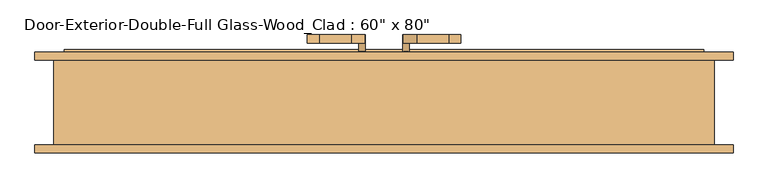
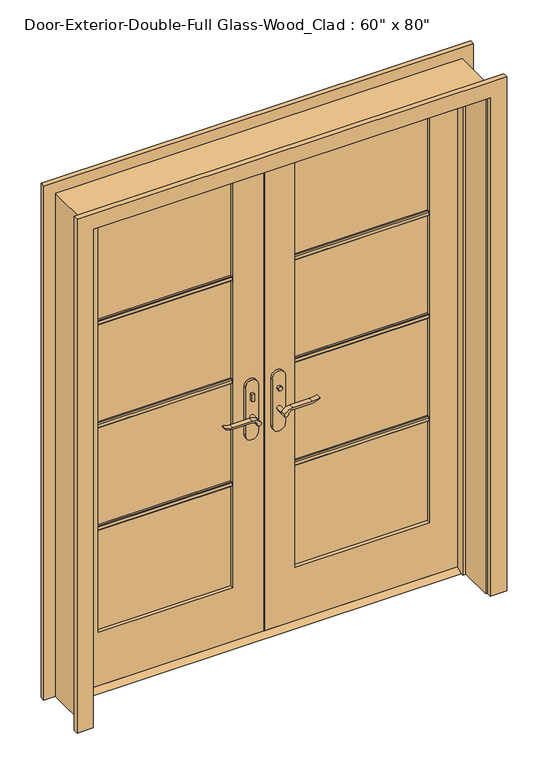
"""IFC4 building model written with IfcOpenShell, lengths in millimetres: door geometry."""

from ifc_helpers import new_model, si_unit, point, frame, frame_2d, origin, place, context, project, spatial, polyline, circle_curve, trimmed, segment, composite_curve, outline, extrude, faceted_brep, source, transform, mapped, element, save


def door_b03bd389(model_context):
    return source(origin(), model_context, "Body", "SolidModel", [
        extrude(outline(polyline([(63.5, 12.7), (98.425, 12.7), (123.825, 0.0), (38.1, 0.0), (63.5, 12.7)])), frame((-762.0, 0.0, 0.0), z_axis=(1.0, 0.0, 0.0), x_axis=(0.0, 1.0, 0.0)), (0.0, 0.0, 1.0), 1524.0),
        extrude(outline(polyline([(-47.4019111, 43.5), (-57.4019111, 43.5), (-57.4019111, 53.5), (-47.4019111, 53.5), (-47.4019111, 43.5)])), frame((0.0, 0.0, 981.9), z_axis=(0.0, 0.0, 1.0), x_axis=(1.0, 0.0, 0.0)), (0.0, 0.0, 1.0), 30.0),
        extrude(outline(composite_curve([segment(trimmed(circle_curve(frame_2d((996.9, -52.4019111)), 8.0), [point((996.9, -60.4019111))], [point((996.9, -44.4019111))], False, "CARTESIAN"), True, "CONTINUOUS"), segment(trimmed(circle_curve(frame_2d((996.9, -52.4019111)), 8.0), [point((996.9, -44.4019111))], [point((996.9, -60.4019111))], False, "CARTESIAN"), True, "CONTINUOUS")], self_intersect=False)), frame((0.0, 108.425, 0.0), z_axis=(0.0, 1.0, 0.0), x_axis=(0.0, 0.0, 1.0)), (0.0, 0.0, 1.0), 10.0),
        extrude(outline(composite_curve([segment(trimmed(circle_curve(frame_2d((897.1555521, -76.0694241)), 37.2832219), [point((919.0523287, -45.8937749))], [point((934.4, -77.7693445))], False, "CARTESIAN"), True, "CONTINUOUS"), segment(polyline([(934.4, -77.7693445), (934.4, -154.045502)]), True, "CONTINUOUS"), segment(trimmed(circle_curve(frame_2d((1017.6850638, -153.9791202)), 83.2850902), [point((934.4, -154.045502))], [point((939.4, -182.4019111))], True, "CARTESIAN"), True, "CONTINUOUS"), segment(polyline([(939.4, -182.4019111), (936.6135558, -182.4019111)]), True, "CONTINUOUS"), segment(trimmed(circle_curve(frame_2d((986.6709207, -150.4622499)), 59.3791355), [point((936.6135558, -182.4019111))], [point((927.4, -154.045502))], False, "CARTESIAN"), True, "CONTINUOUS"), segment(polyline([(927.4, -154.045502), (927.4, -77.7881013)]), True, "CONTINUOUS"), segment(trimmed(circle_curve(frame_2d((909.2738613, -77.7881013)), 18.1261387), [point((927.4, -77.7881013))], [point((914.4, -60.4019111))], True, "CARTESIAN"), True, "CONTINUOUS"), segment(trimmed(circle_curve(frame_2d((914.4, -52.4019111)), 8.0), [point((914.4, -60.4019111))], [point((919.0523287, -45.8937749))], False, "CARTESIAN"), True, "CONTINUOUS")], self_intersect=False)), frame((0.0, 3.5, 0.0), z_axis=(0.0, 1.0, 0.0), x_axis=(0.0, 0.0, 1.0)), (0.0, 0.0, 1.0), 20.0),
        extrude(outline(composite_curve([segment(trimmed(circle_curve(frame_2d((914.4, -52.4019111)), 8.0), [point((914.3999903, -60.4019111))], [point((919.0523287, -45.8937749))], False, "CARTESIAN"), True, "CONTINUOUS"), segment(trimmed(circle_curve(frame_2d((897.1555521, -76.0694241)), 37.2832219), [point((919.0523287, -45.8937749))], [point((934.4, -77.7693445))], False, "CARTESIAN"), True, "CONTINUOUS"), segment(polyline([(934.4, -77.7693445), (934.4, -154.045502)]), True, "CONTINUOUS"), segment(trimmed(circle_curve(frame_2d((1017.6850638, -153.9791202)), 83.2850902), [point((934.4, -154.045502))], [point((939.4, -182.4019111))], True, "CARTESIAN"), True, "CONTINUOUS"), segment(polyline([(939.4, -182.4019111), (936.6135558, -182.4019111)]), True, "CONTINUOUS"), segment(trimmed(circle_curve(frame_2d((986.6709207, -150.4622499)), 59.3791355), [point((936.6135558, -182.4019111))], [point((927.4, -154.045502))], False, "CARTESIAN"), True, "CONTINUOUS"), segment(polyline([(927.4, -154.045502), (927.4, -77.788099)]), True, "CONTINUOUS"), segment(trimmed(circle_curve(frame_2d((909.2738682, -77.788099)), 18.1261318), [point((927.4, -77.788099))], [point((914.3999903, -60.4019111))], True, "CARTESIAN"), True, "CONTINUOUS")], self_intersect=False)), frame((0.0, 138.425, 0.0), z_axis=(0.0, 1.0, 0.0), x_axis=(0.0, 0.0, 1.0)), (0.0, 0.0, 1.0), 20.0),
        extrude(outline(composite_curve([segment(trimmed(circle_curve(frame_2d((914.4, -52.4019111)), 8.0), [point((914.4, -60.4019111))], [point((914.4, -44.4019111))], False, "CARTESIAN"), True, "CONTINUOUS"), segment(trimmed(circle_curve(frame_2d((914.4, -52.4019111)), 8.0), [point((914.4, -44.4019111))], [point((914.4, -60.4019111))], False, "CARTESIAN"), True, "CONTINUOUS")], self_intersect=False)), frame((0.0, 23.5, 0.0), z_axis=(0.0, 1.0, 0.0), x_axis=(0.0, 0.0, 1.0)), (0.0, 0.0, 1.0), 30.0),
        extrude(outline(composite_curve([segment(trimmed(circle_curve(frame_2d((914.4, -52.4019111)), 8.0), [point((914.4, -60.4019111))], [point((914.4, -44.4019111))], False, "CARTESIAN"), True, "CONTINUOUS"), segment(trimmed(circle_curve(frame_2d((914.4, -52.4019111)), 8.0), [point((914.4, -44.4019111))], [point((914.4, -60.4019111))], False, "CARTESIAN"), True, "CONTINUOUS")], self_intersect=False)), frame((0.0, 108.425, 0.0), z_axis=(0.0, 1.0, 0.0), x_axis=(0.0, 0.0, 1.0)), (0.0, 0.0, 1.0), 30.0),
        extrude(outline(composite_curve([segment(polyline([(844.4, -27.4019111), (1039.4, -27.4019111)]), True, "CONTINUOUS"), segment(trimmed(circle_curve(frame_2d((1039.4, -52.4019111)), 25.0), [point((1039.4, -27.4019111))], [point((1039.4, -77.4019111))], False, "CARTESIAN"), True, "CONTINUOUS"), segment(polyline([(1039.4, -77.4019111), (844.4, -77.4019111)]), True, "CONTINUOUS"), segment(trimmed(circle_curve(frame_2d((844.4, -52.4019111)), 25.0), [point((844.4, -77.4019111))], [point((844.4, -27.4019111))], False, "CARTESIAN"), True, "CONTINUOUS")], self_intersect=False)), frame((0.0, 53.5, 0.0), z_axis=(0.0, 1.0, 0.0), x_axis=(0.0, 0.0, 1.0)), (0.0, 0.0, 1.0), 10.0),
        extrude(outline(composite_curve([segment(polyline([(844.4, -27.4019111), (1039.4, -27.4019111)]), True, "CONTINUOUS"), segment(trimmed(circle_curve(frame_2d((1039.4, -52.4019111)), 25.0), [point((1039.4, -27.4019111))], [point((1039.4, -77.4019111))], False, "CARTESIAN"), True, "CONTINUOUS"), segment(polyline([(1039.4, -77.4019111), (844.4, -77.4019111)]), True, "CONTINUOUS"), segment(trimmed(circle_curve(frame_2d((844.4, -52.4019111)), 25.0), [point((844.4, -77.4019111))], [point((844.4, -27.4019111))], False, "CARTESIAN"), True, "CONTINUOUS")], self_intersect=False)), frame((0.0, 98.425, 0.0), z_axis=(0.0, 1.0, 0.0), x_axis=(0.0, 0.0, 1.0)), (0.0, 0.0, 1.0), 10.0),
        extrude(outline(polyline([(47.3875, 118.425), (57.3875, 118.425), (57.3875, 108.425), (47.3875, 108.425), (47.3875, 118.425)])), frame((0.0, 0.0, 981.9), z_axis=(0.0, 0.0, 1.0), x_axis=(1.0, 0.0, 0.0)), (0.0, 0.0, 1.0), 30.0),
        extrude(outline(composite_curve([segment(trimmed(circle_curve(frame_2d((996.9, 52.3875)), 8.0), [point((996.9, 60.3875))], [point((996.9, 44.3875))], False, "CARTESIAN"), True, "CONTINUOUS"), segment(trimmed(circle_curve(frame_2d((996.9, 52.3875)), 8.0), [point((996.9, 44.3875))], [point((996.9, 60.3875))], False, "CARTESIAN"), True, "CONTINUOUS")], self_intersect=False)), frame((0.0, 43.5, 0.0), z_axis=(0.0, 1.0, 0.0), x_axis=(0.0, 0.0, 1.0)), (0.0, 0.0, 1.0), 10.0),
        extrude(outline(composite_curve([segment(trimmed(circle_curve(frame_2d((914.4, 52.3875)), 8.0), [point((919.0523287, 45.8793637))], [point((914.4, 60.3875))], False, "CARTESIAN"), True, "CONTINUOUS"), segment(trimmed(circle_curve(frame_2d((909.2738613, 77.7736901)), 18.1261387), [point((914.4, 60.3875))], [point((927.4, 77.7736901))], True, "CARTESIAN"), True, "CONTINUOUS"), segment(polyline([(927.4, 77.7736901), (927.4, 154.0310909)]), True, "CONTINUOUS"), segment(trimmed(circle_curve(frame_2d((986.6709207, 150.4478388)), 59.3791355), [point((927.4, 154.0310909))], [point((936.6135558, 182.3875))], False, "CARTESIAN"), True, "CONTINUOUS"), segment(polyline([(936.6135558, 182.3875), (939.4, 182.3875)]), True, "CONTINUOUS"), segment(trimmed(circle_curve(frame_2d((1017.6850638, 153.9647091)), 83.2850902), [point((939.4, 182.3875))], [point((934.4, 154.0310909))], True, "CARTESIAN"), True, "CONTINUOUS"), segment(polyline([(934.4, 154.0310909), (934.4, 77.7549333)]), True, "CONTINUOUS"), segment(trimmed(circle_curve(frame_2d((897.1555521, 76.0550129)), 37.2832219), [point((934.4, 77.7549333))], [point((919.0523287, 45.8793637))], False, "CARTESIAN"), True, "CONTINUOUS")], self_intersect=False)), frame((0.0, 138.425, 0.0), z_axis=(0.0, 1.0, 0.0), x_axis=(0.0, 0.0, 1.0)), (0.0, 0.0, 1.0), 20.0),
        extrude(outline(composite_curve([segment(trimmed(circle_curve(frame_2d((909.2738682, 77.7736878)), 18.1261318), [point((914.3999903, 60.3875))], [point((927.4, 77.7736878))], True, "CARTESIAN"), True, "CONTINUOUS"), segment(polyline([(927.4, 77.7736878), (927.4, 154.0310909)]), True, "CONTINUOUS"), segment(trimmed(circle_curve(frame_2d((986.6709207, 150.4478388)), 59.3791355), [point((927.4, 154.0310909))], [point((936.6135558, 182.3875))], False, "CARTESIAN"), True, "CONTINUOUS"), segment(polyline([(936.6135558, 182.3875), (939.4, 182.3875)]), True, "CONTINUOUS"), segment(trimmed(circle_curve(frame_2d((1017.6850638, 153.9647091)), 83.2850902), [point((939.4, 182.3875))], [point((934.4, 154.0310909))], True, "CARTESIAN"), True, "CONTINUOUS"), segment(polyline([(934.4, 154.0310909), (934.4, 77.7549333)]), True, "CONTINUOUS"), segment(trimmed(circle_curve(frame_2d((897.1555521, 76.0550129)), 37.2832219), [point((934.4, 77.7549333))], [point((919.0523287, 45.8793637))], False, "CARTESIAN"), True, "CONTINUOUS"), segment(trimmed(circle_curve(frame_2d((914.4, 52.3875)), 8.0), [point((919.0523287, 45.8793637))], [point((914.3999903, 60.3875))], False, "CARTESIAN"), True, "CONTINUOUS")], self_intersect=False)), frame((0.0, 3.5, 0.0), z_axis=(0.0, 1.0, 0.0), x_axis=(0.0, 0.0, 1.0)), (0.0, 0.0, 1.0), 20.0),
        extrude(outline(composite_curve([segment(trimmed(circle_curve(frame_2d((914.4, 52.3875)), 8.0), [point((914.4, 60.3875))], [point((914.4, 44.3875))], False, "CARTESIAN"), True, "CONTINUOUS"), segment(trimmed(circle_curve(frame_2d((914.4, 52.3875)), 8.0), [point((914.4, 44.3875))], [point((914.4, 60.3875))], False, "CARTESIAN"), True, "CONTINUOUS")], self_intersect=False)), frame((0.0, 108.425, 0.0), z_axis=(0.0, 1.0, 0.0), x_axis=(0.0, 0.0, 1.0)), (0.0, 0.0, 1.0), 30.0),
        extrude(outline(composite_curve([segment(trimmed(circle_curve(frame_2d((914.4, 52.3875)), 8.0), [point((914.4, 60.3875))], [point((914.4, 44.3875))], False, "CARTESIAN"), True, "CONTINUOUS"), segment(trimmed(circle_curve(frame_2d((914.4, 52.3875)), 8.0), [point((914.4, 44.3875))], [point((914.4, 60.3875))], False, "CARTESIAN"), True, "CONTINUOUS")], self_intersect=False)), frame((0.0, 23.5, 0.0), z_axis=(0.0, 1.0, 0.0), x_axis=(0.0, 0.0, 1.0)), (0.0, 0.0, 1.0), 30.0),
        extrude(outline(composite_curve([segment(trimmed(circle_curve(frame_2d((844.4, 52.3875)), 25.0), [point((844.4, 27.3875))], [point((844.4, 77.3875))], False, "CARTESIAN"), True, "CONTINUOUS"), segment(polyline([(844.4, 77.3875), (1039.4, 77.3875)]), True, "CONTINUOUS"), segment(trimmed(circle_curve(frame_2d((1039.4, 52.3875)), 25.0), [point((1039.4, 77.3875))], [point((1039.4, 27.3875))], False, "CARTESIAN"), True, "CONTINUOUS"), segment(polyline([(1039.4, 27.3875), (844.4, 27.3875)]), True, "CONTINUOUS")], self_intersect=False)), frame((0.0, 98.425, 0.0), z_axis=(0.0, 1.0, 0.0), x_axis=(0.0, 0.0, 1.0)), (0.0, 0.0, 1.0), 10.0),
        extrude(outline(composite_curve([segment(trimmed(circle_curve(frame_2d((844.4, 52.3875)), 25.0), [point((844.4, 27.3875))], [point((844.4, 77.3875))], False, "CARTESIAN"), True, "CONTINUOUS"), segment(polyline([(844.4, 77.3875), (1039.4, 77.3875)]), True, "CONTINUOUS"), segment(trimmed(circle_curve(frame_2d((1039.4, 52.3875)), 25.0), [point((1039.4, 77.3875))], [point((1039.4, 27.3875))], False, "CARTESIAN"), True, "CONTINUOUS"), segment(polyline([(1039.4, 27.3875), (844.4, 27.3875)]), True, "CONTINUOUS")], self_intersect=False)), frame((0.0, 53.5, 0.0), z_axis=(0.0, 1.0, 0.0), x_axis=(0.0, 0.0, 1.0)), (0.0, 0.0, 1.0), 10.0),
        extrude(outline(polyline([(77.47, 1502.171875), (77.47, 1483.121875), (71.12, 1483.121875), (67.945, 1486.296875), (67.945, 1498.996875), (71.12, 1502.171875), (77.47, 1502.171875)])), frame((120.65, 0.0, 0.0), z_axis=(1.0, 0.0, 0.0), x_axis=(0.0, 1.0, 0.0)), (0.0, 0.0, 1.0), 520.7),
        extrude(outline(polyline([(77.47, 1081.88125), (77.47, 1062.83125), (71.12, 1062.83125), (67.945, 1066.00625), (67.945, 1078.70625), (71.12, 1081.88125), (77.47, 1081.88125)])), frame((120.65, 0.0, 0.0), z_axis=(1.0, 0.0, 0.0), x_axis=(0.0, 1.0, 0.0)), (0.0, 0.0, 1.0), 520.7),
        extrude(outline(polyline([(77.47, 661.590625), (77.47, 642.540625), (71.12, 642.540625), (67.945, 645.715625), (67.945, 658.415625), (71.12, 661.590625), (77.47, 661.590625)])), frame((120.65, 0.0, 0.0), z_axis=(1.0, 0.0, 0.0), x_axis=(0.0, 1.0, 0.0)), (0.0, 0.0, 1.0), 520.7),
        extrude(outline(polyline([(84.455, 1502.171875), (90.805, 1502.171875), (93.98, 1498.996875), (93.98, 1486.296875), (90.805, 1483.121875), (84.455, 1483.121875), (84.455, 1502.171875)])), frame((-641.35, 0.0, 0.0), z_axis=(1.0, 0.0, 0.0), x_axis=(0.0, 1.0, 0.0)), (0.0, 0.0, 1.0), 520.7),
        extrude(outline(polyline([(84.455, 1081.88125), (90.805, 1081.88125), (93.98, 1078.70625), (93.98, 1066.00625), (90.805, 1062.83125), (84.455, 1062.83125), (84.455, 1081.88125)])), frame((-641.35, 0.0, 0.0), z_axis=(1.0, 0.0, 0.0), x_axis=(0.0, 1.0, 0.0)), (0.0, 0.0, 1.0), 520.7),
        extrude(outline(polyline([(84.455, 661.590625), (90.805, 661.590625), (93.98, 658.415625), (93.98, 645.715625), (90.805, 642.540625), (84.455, 642.540625), (84.455, 661.590625)])), frame((-641.35, 0.0, 0.0), z_axis=(1.0, 0.0, 0.0), x_axis=(0.0, 1.0, 0.0)), (0.0, 0.0, 1.0), 520.7),
        extrude(outline(polyline([(84.455, 1502.171875), (90.805, 1502.171875), (93.98, 1498.996875), (93.98, 1486.296875), (90.805, 1483.121875), (84.455, 1483.121875), (84.455, 1502.171875)])), frame((120.65, 0.0, 0.0), z_axis=(1.0, 0.0, 0.0), x_axis=(0.0, 1.0, 0.0)), (0.0, 0.0, 1.0), 520.7),
        extrude(outline(polyline([(84.455, 1081.88125), (90.805, 1081.88125), (93.98, 1078.70625), (93.98, 1066.00625), (90.805, 1062.83125), (84.455, 1062.83125), (84.455, 1081.88125)])), frame((120.65, 0.0, 0.0), z_axis=(1.0, 0.0, 0.0), x_axis=(0.0, 1.0, 0.0)), (0.0, 0.0, 1.0), 520.7),
        extrude(outline(polyline([(84.455, 661.590625), (90.805, 661.590625), (93.98, 658.415625), (93.98, 645.715625), (90.805, 642.540625), (84.455, 642.540625), (84.455, 661.590625)])), frame((120.65, 0.0, 0.0), z_axis=(1.0, 0.0, 0.0), x_axis=(0.0, 1.0, 0.0)), (0.0, 0.0, 1.0), 520.7),
        extrude(outline(polyline([(77.47, 1502.171875), (77.47, 1483.121875), (71.12, 1483.121875), (67.945, 1486.296875), (67.945, 1498.996875), (71.12, 1502.171875), (77.47, 1502.171875)])), frame((-641.35, 0.0, 0.0), z_axis=(1.0, 0.0, 0.0), x_axis=(0.0, 1.0, 0.0)), (0.0, 0.0, 1.0), 520.7),
        extrude(outline(polyline([(77.47, 1081.88125), (77.47, 1062.83125), (71.12, 1062.83125), (67.945, 1066.00625), (67.945, 1078.70625), (71.12, 1081.88125), (77.47, 1081.88125)])), frame((-641.35, 0.0, 0.0), z_axis=(1.0, 0.0, 0.0), x_axis=(0.0, 1.0, 0.0)), (0.0, 0.0, 1.0), 520.7),
        extrude(outline(polyline([(77.47, 661.590625), (77.47, 642.540625), (71.12, 642.540625), (67.945, 645.715625), (67.945, 658.415625), (71.12, 661.590625), (77.47, 661.590625)])), frame((-641.35, 0.0, 0.0), z_axis=(1.0, 0.0, 0.0), x_axis=(0.0, 1.0, 0.0)), (0.0, 0.0, 1.0), 520.7),
        extrude(outline(polyline([(0.0, 768.35), (0.0, 831.85), (2101.85, 831.85), (2101.85, -831.85), (0.0, -831.85), (0.0, -768.35), (2038.35, -768.35), (2038.35, 768.35), (0.0, 768.35)])), frame((0.0, 98.425, 0.0), z_axis=(0.0, 1.0, 0.0), x_axis=(0.0, 0.0, 1.0)), (0.0, 0.0, 1.0), 19.05),
        extrude(outline(polyline([(0.0, 768.35), (0.0, 831.85), (2101.85, 831.85), (2101.85, -831.85), (0.0, -831.85), (0.0, -768.35), (2038.35, -768.35), (2038.35, 768.35), (0.0, 768.35)])), frame((0.0, -123.825, 0.0), z_axis=(0.0, 1.0, 0.0), x_axis=(0.0, 0.0, 1.0)), (0.0, 0.0, 1.0), 19.05),
        extrude(outline(polyline([(12.7, 762.0), (2032.0, 762.0), (2032.0, 1.5875), (12.7, 1.5875), (12.7, 762.0)]), holes=[polyline([(1912.9375, 120.65), (1912.9375, 641.35), (231.775, 641.35), (231.775, 120.65), (1912.9375, 120.65)])]), frame((0.0, 63.5, 0.0), z_axis=(0.0, 1.0, 0.0), x_axis=(0.0, 0.0, 1.0)), (0.0, 0.0, 1.0), 34.925),
        extrude(outline(polyline([(2032.0, -762.0), (12.7, -762.0), (12.7, -1.6019111), (2032.0, -1.6019111), (2032.0, -762.0)]), holes=[polyline([(231.775, -641.35), (1912.9375, -641.35), (1912.9375, -120.65), (231.775, -120.65), (231.775, -641.35)])]), frame((0.0, 63.5, 0.0), z_axis=(0.0, 1.0, 0.0), x_axis=(0.0, 0.0, 1.0)), (0.0, 0.0, 1.0), 34.925),
        faceted_brep([(787.4, 98.425, 0.0), (787.4, -104.775, 0.0), (762.0, -104.775, 0.0), (762.0, 28.575, 0.0), (749.3, 28.575, 0.0), (749.3, 63.5, 0.0), (762.0, 63.5, 0.0), (762.0, 98.425, 0.0), (787.4, 98.425, 2057.4), (787.4, -104.775, 2057.4), (-787.4, -104.775, 2057.4), (-787.4, -104.775, 0.0), (-762.0, -104.775, 0.0), (-762.0, -104.775, 2032.0), (762.0, -104.775, 2032.0), (762.0, 28.575, 2032.0), (-762.0, 28.575, 2032.0), (-762.0, 28.575, 0.0), (-749.3, 28.575, 0.0), (-749.3, 28.575, 2019.3), (749.3, 28.575, 2019.3), (749.3, 63.5, 2019.3), (1.5875, 63.5, 2019.3), (-1.6019111, 63.5, 2019.3), (-749.3, 63.5, 2019.3), (-749.3, 63.5, 0.0), (-762.0, 63.5, 0.0), (-762.0, 63.5, 2032.0), (-1.6019111, 63.5, 2032.0), (1.5875, 63.5, 2032.0), (762.0, 63.5, 2032.0), (762.0, 98.425, 2032.0), (1.5875, 98.425, 2032.0), (-1.6019111, 98.425, 2032.0), (-762.0, 98.425, 2032.0), (-762.0, 98.425, 0.0), (-787.4, 98.425, 0.0), (-787.4, 98.425, 2057.4)], [[[0, 1, 2, 3, 4, 5, 6, 7]], [[1, 0, 8, 9]], [[2, 1, 9, 10, 11, 12, 13, 14]], [[3, 2, 14, 15]], [[4, 3, 15, 16, 17, 18, 19, 20]], [[5, 4, 20, 21]], [[6, 5, 21, 22, 23, 24, 25, 26, 27, 28, 29, 30]], [[7, 6, 30, 31]], [[0, 7, 31, 32, 33, 34, 35, 36, 37, 8]], [[9, 8, 37, 10]], [[14, 13, 16, 15]], [[20, 19, 24, 23, 22, 21]], [[31, 30, 29, 28, 27, 34, 33, 32]], [[12, 11, 36, 35, 26, 25, 18, 17]], [[11, 10, 37, 36]], [[13, 12, 17, 16]], [[19, 18, 25, 24]], [[27, 26, 35, 34]]]),
        extrude(outline(polyline([(641.35, 77.47), (120.65, 77.47), (120.65, 84.455), (641.35, 84.455), (641.35, 77.47)])), frame((0.0, 0.0, 231.775), z_axis=(0.0, 0.0, 1.0), x_axis=(1.0, 0.0, 0.0)), (0.0, 0.0, 1.0), 1681.1625),
        extrude(outline(polyline([(-120.65, 77.47), (-641.35, 77.47), (-641.35, 84.455), (-120.65, 84.455), (-120.65, 77.47)])), frame((0.0, 0.0, 231.775), z_axis=(0.0, 0.0, 1.0), x_axis=(1.0, 0.0, 0.0)), (0.0, 0.0, 1.0), 1681.1625),
    ])


if __name__ == "__main__":
    model = new_model("IFC4")
    model_context = context("Model", 3, world=origin())
    ifc_project = project(units=[si_unit("LENGTHUNIT", "METRE", prefix="MILLI")], contexts=[model_context])
    site = spatial("IfcSite", under=ifc_project)
    building = spatial("IfcBuilding", under=site)
    placement = place(None, origin())
    door_shape = door_b03bd389(model_context)
    element("IfcDoor", 1, ObjectType="Door-Exterior-Double-Full Glass-Wood_Clad : 60\" x 80\"", at=placement, inside=building, context=model_context, shape_type="MappedRepresentation", body=[
        mapped(door_shape, transform((0.0, 0.0, 0.0), x_axis=(1.0, 0.0, 0.0), y_axis=(0.0, 1.0, 0.0), z_axis=(0.0, 0.0, 1.0))),
    ])
    save(model, "model.ifc")

# Revit data of these elements
# Type "Door-Exterior-Double-Full Glass-Wood_Clad : 60\" x 80\""
#   Type Mark = "15"
#   Assembly Code = "B2030100"
#   Analytic Construction = "French door, wood frame with double glass"
#   Top Rail = 0' - 4 11/16"
#   Threshold Offset [instance default] = 0' - 0 1/2"
#   Thickness = 0' - 1 3/8"
#   Thermal Resistance (R) = 1.9158 (h·ft²·°F)/BTU
#   Swing Angle [instance default] = 90.00°
#   Stiles = 0' - 4 3/4"
#   Rough Width = 5' - 2"
#   Rough Height = 6' - 9"
#   Panel Width = 2' - 6"
#   Door Offset [instance default] = 0' - 0"
#   Height = 6' - 8"
#   Width = 5' - 0"
#   Heat Transfer Coefficient (U) = 0.5220 BTU/(h·ft²·°F)
#   Bottom Rail = 0' - 9 1/8"
#   Exterior Trim [instance default] = yes
#   Threshold [instance default] = yes
#   Show Grill [instance default] = yes
#   Function = 1
#   Trim Material = Cherry
#   Threshold Material = Cherry
#   Panel Material = Cherry
#   Glazing = Glass
#   Frame Material = Cherry
#   Door Handle Material = Aluminum
#   Visual Light Transmittance = 0
#   Solar Heat Gain Coefficient = 0
#   Wall Closure = (empty or 0)
#   Construction Type = (empty or 0)
# Element 1 (IfcDoor, "Door-Exterior-Double-Full Glass-Wood_Clad : 60\" x 80\"")
#   Materials on its faces: "Cherry", "Aluminum", "Glass"
# Materials
#   "Cherry": class "Wood", colour RGB 226 177 128, transparency 0, Description = "Prunus Serotina", Cost = 0
#   "Glass": class "Glass", colour RGB 0 128 192, transparency 0.75, Description = "Soda Lime Glass", Cost = 0
#   "Aluminum": class "Metal", colour RGB 247 247 247, transparency 0, Description = "Aluminum 6061", Cost = 0
